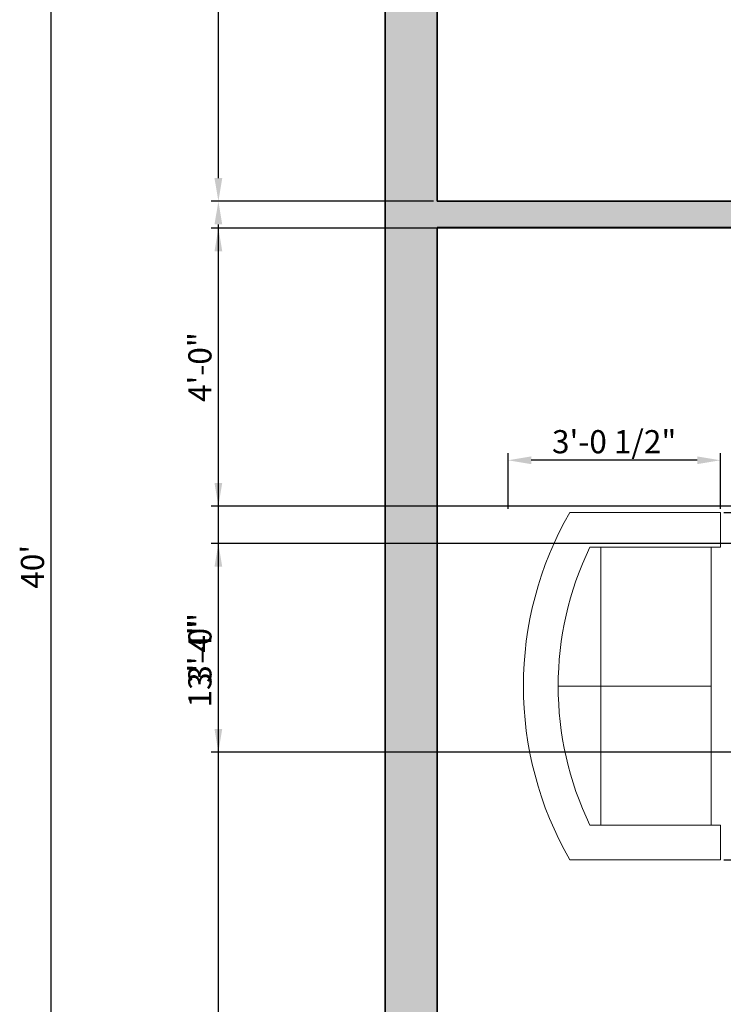
# Model space of a CAD drawing. Units: inches. Extents: x 1872 to 2380, y 714 to 1327.
# Tile 4 of 9: x 1872 to 1994, y 974 to 1144. Entities that reach past the tile are written whole.
import ezdxf

# ---------------------------------------------------------------- set-up
doc = ezdxf.new("R2010")
doc.units = ezdxf.units.IN
for name, color, linetype, lineweight in [('A-ANNO-DIMS', 2, 'Continuous', 18), ('A-FURN', 8, 'Continuous', 18), ('A-WALL', 7, 'Continuous', 35)]:
    doc.layers.add(name, color=color, linetype=linetype, lineweight=lineweight)
doc.layers.add('A-WALL-PATT', color=242, linetype='Continuous', lineweight=13, true_color=0xd52e31)
doc.styles.get("Standard").update_dxf_attribs({"font": 'arial.ttf'})
doc.dimstyles.new('ISO-25', dxfattribs={"dimtxt": 4, "dimasz": 4, "dimexe": 1.25, "dimexo": 0.625, "dimtad": 1, "dimdec": 0, "dimlunit": 3, "dimtxsty": 'Standard', "dimcen": 2.5, "dimadec": 0, "dimazin": 0, "dimtfac": 1, "dimtdec": 0, "dimtmove": 0, "dimatfit": 3, "dimfxl": 1, "dimarcsym": 0})

# ---------------------------------------------------------------- blocks, each defined once
blk = doc.blocks.new('Sofa - Roundback Loveseat 5 ft.')
for p, q in [((0, -32.44198), (0, -5.99998)), ((-24, -33.99998), (-24, -11.46958)), ((24.00004, -33.99998), (24.00004, -11.46958)), ((-23.9998, -13.38178), (23.99986, -13.38178)), ((-24, -32.44198), (24.00004, -32.44198))]:
    blk.add_line(p, q)
for points in [[(-24, -33.99998), (-30, -33.99998), (-30, -7.99998)], [(30.00004, -7.99998), (30.00004, -33.99998), (24.00004, -33.99998)]]:
    blk.add_lwpolyline(points)
for centre, radius, start, end in [((0, -60.24998), 60.24998, 60.13715, 119.8628), ((0, -61.38438), 55.38444, 64.32083, 115.6792)]:
    blk.add_arc(centre, radius, start, end)
blk = doc.blocks.new('*D23')
at = {"layer": 'A-ANNO-DIMS', "color": 0, "lineweight": -2, "transparency": 16777216}
for p, q in [((1934.77, 1289.64), (1876.44, 1289.64)), ((1877.69, 1285.64), (1877.69, 813.64)), ((1934.77, 809.64), (1876.44, 809.64))]:
    blk.add_line(p, q, dxfattribs=at)
at = {"layer": 'A-ANNO-DIMS', "color": 0, "transparency": 16777216}
for points in [[(1877.02, 1285.64), (1878.36, 1285.64), (1877.69, 1289.64)], [(1877.02, 813.64), (1878.36, 813.64), (1877.69, 809.64)]]:
    blk.add_solid(points, dxfattribs=at)
at = {"layer": 'Defpoints', "color": 0, "transparency": 16777216}
for p in [(1935.4, 1289.64), (1877.69, 809.64), (1935.4, 809.64)]:
    blk.add_point(p, dxfattribs=at)
at = {"layer": 'A-ANNO-DIMS', "color": 0, "transparency": 16777216, "insert": (1875.02, 1049.64), "char_height": 4, "attachment_point": 5, "rotation": 90}
blk.add_mtext("40'", dxfattribs=at)
blk = doc.blocks.new('*D40')
at = {"layer": 'A-ANNO-DIMS', "color": 0, "lineweight": -2, "transparency": 16777216}
for p, q in [((1993.9, 1059.04), (2003.52, 1059.04)), ((2002.27, 1003.04), (2002.27, 1055.04)), ((1993.9, 999.04), (2003.52, 999.04))]:
    blk.add_line(p, q, dxfattribs=at)
at = {"layer": 'A-ANNO-DIMS', "color": 0, "transparency": 16777216}
for points in [[(2001.61, 1055.04), (2002.94, 1055.04), (2002.27, 1059.04)], [(2001.61, 1003.04), (2002.94, 1003.04), (2002.27, 999.04)]]:
    blk.add_solid(points, dxfattribs=at)
at = {"layer": 'Defpoints', "color": 0, "transparency": 16777216}
for p in [(1993.27, 1059.04), (2002.27, 1059.04), (1993.27, 999.04)]:
    blk.add_point(p, dxfattribs=at)
at = {"layer": 'A-ANNO-DIMS', "color": 0, "transparency": 16777216, "insert": (1999.58, 1029.04), "char_height": 4, "attachment_point": 5, "rotation": 90}
blk.add_mtext('LOVESEAT 5\'-0"', dxfattribs=at)
blk = doc.blocks.new('*D41')
at = {"layer": 'A-ANNO-DIMS', "color": 0, "lineweight": -2, "transparency": 16777216}
for p, q in [((1956.61, 1059.66), (1956.61, 1069.29)), ((1993.27, 1059.66), (1993.27, 1069.29)), ((1989.27, 1068.04), (1960.61, 1068.04))]:
    blk.add_line(p, q, dxfattribs=at)
at = {"layer": 'A-ANNO-DIMS', "color": 0, "transparency": 16777216}
for points in [[(1960.61, 1068.71), (1960.61, 1067.37), (1956.61, 1068.04)], [(1989.27, 1068.71), (1989.27, 1067.37), (1993.27, 1068.04)]]:
    blk.add_solid(points, dxfattribs=at)
at = {"layer": 'Defpoints', "color": 0, "transparency": 16777216}
for p in [(1956.61, 1068.04), (1956.61, 1059.04), (1993.27, 1059.04)]:
    blk.add_point(p, dxfattribs=at)
at = {"layer": 'A-ANNO-DIMS', "color": 0, "transparency": 16777216, "insert": (1974.94, 1070.73), "char_height": 4, "attachment_point": 5}
blk.add_mtext('3\'-0 1/2"', dxfattribs=at)
blk = doc.blocks.new('*D67')
at = {"layer": 'A-ANNO-DIMS', "color": 0, "lineweight": -2, "transparency": 16777216}
for p, q in [((1943.77, 1112.77), (1905.35, 1112.77)), ((1906.6, 956.99), (1906.6, 1108.77)), ((2000.77, 952.99), (1905.35, 952.99))]:
    blk.add_line(p, q, dxfattribs=at)
at = {"layer": 'A-ANNO-DIMS', "color": 0, "transparency": 16777216}
for points in [[(1905.93, 1108.77), (1907.27, 1108.77), (1906.6, 1112.77)], [(1905.93, 956.99), (1907.27, 956.99), (1906.6, 952.99)]]:
    blk.add_solid(points, dxfattribs=at)
at = {"layer": 'Defpoints', "color": 0, "transparency": 16777216}
for p in [(1906.6, 1112.77), (1944.4, 1112.77), (2001.4, 952.99)]:
    blk.add_point(p, dxfattribs=at)
at = {"layer": 'A-ANNO-DIMS', "color": 0, "transparency": 16777216, "insert": (1903.93, 1032.88), "char_height": 4, "attachment_point": 5, "rotation": 90}
blk.add_mtext('13\'-4"', dxfattribs=at)
blk = doc.blocks.new('*D68')
at = {"layer": 'A-ANNO-DIMS', "color": 0, "lineweight": -2, "transparency": 16777216}
for p, q in [((1934.77, 1289.64), (1905.35, 1289.64)), ((1906.6, 1116.77), (1906.6, 1285.64)), ((1943.77, 1112.77), (1905.35, 1112.77))]:
    blk.add_line(p, q, dxfattribs=at)
at = {"layer": 'A-ANNO-DIMS', "color": 0, "transparency": 16777216}
for points in [[(1905.93, 1285.64), (1907.27, 1285.64), (1906.6, 1289.64)], [(1905.93, 1116.77), (1907.27, 1116.77), (1906.6, 1112.77)]]:
    blk.add_solid(points, dxfattribs=at)
at = {"layer": 'Defpoints', "color": 0, "transparency": 16777216}
for p in [(1906.6, 1289.64), (1935.4, 1289.64), (1944.4, 1112.77)]:
    blk.add_point(p, dxfattribs=at)
at = {"layer": 'A-ANNO-DIMS', "color": 0, "transparency": 16777216, "insert": (1903.93, 1201.21), "char_height": 4, "attachment_point": 5, "rotation": 90}
blk.add_mtext('14\'-9"', dxfattribs=at)
blk = doc.blocks.new('*D72')
at = {"layer": 'A-ANNO-DIMS', "color": 0, "lineweight": -2, "transparency": 16777216}
for p, q in [((2197.27, 1108.14), (1905.35, 1108.14)), ((1906.6, 1064.14), (1906.6, 1104.14)), ((2197.27, 1060.14), (1905.35, 1060.14))]:
    blk.add_line(p, q, dxfattribs=at)
at = {"layer": 'A-ANNO-DIMS', "color": 0, "transparency": 16777216}
for points in [[(1905.93, 1104.14), (1907.27, 1104.14), (1906.6, 1108.14)], [(1905.93, 1064.14), (1907.27, 1064.14), (1906.6, 1060.14)]]:
    blk.add_solid(points, dxfattribs=at)
at = {"layer": 'Defpoints', "color": 0, "transparency": 16777216}
for p in [(1906.6, 1108.14), (2197.9, 1108.14), (2197.9, 1060.14)]:
    blk.add_point(p, dxfattribs=at)
at = {"layer": 'A-ANNO-DIMS', "color": 0, "transparency": 16777216, "insert": (1903.93, 1084.14), "char_height": 4, "attachment_point": 5, "rotation": 90}
blk.add_mtext('4\'-0"', dxfattribs=at)
blk = doc.blocks.new('*D73')
at = {"layer": 'A-ANNO-DIMS', "color": 0, "lineweight": -2, "transparency": 16777216}
for p, q in [((2197.27, 1053.64), (1905.35, 1053.64)), ((1906.6, 1021.64), (1906.6, 1049.64)), ((2197.27, 1017.64), (1905.35, 1017.64))]:
    blk.add_line(p, q, dxfattribs=at)
at = {"layer": 'A-ANNO-DIMS', "color": 0, "transparency": 16777216}
for points in [[(1905.93, 1049.64), (1907.27, 1049.64), (1906.6, 1053.64)], [(1905.93, 1021.64), (1907.27, 1021.64), (1906.6, 1017.64)]]:
    blk.add_solid(points, dxfattribs=at)
at = {"layer": 'Defpoints', "color": 0, "transparency": 16777216}
for p in [(1906.6, 1053.64), (2197.9, 1053.64), (2197.9, 1017.64)]:
    blk.add_point(p, dxfattribs=at)
at = {"layer": 'A-ANNO-DIMS', "color": 0, "transparency": 16777216, "insert": (1903.93, 1035.64), "char_height": 4, "attachment_point": 5, "rotation": 90}
blk.add_mtext('3\'-0"', dxfattribs=at)

msp = doc.modelspace()

# ---------------------------------------------------------------- hatches: boundary and pattern name
at = {"layer": 'A-WALL-PATT', "transparency": 33554687}
h = msp.add_hatch(color=256, dxfattribs=at)
h.dxf.hatch_style = 1
h.paths.add_polyline_path([(2295.4, 1289.64), (1935.4, 1289.64), (1935.4, 809.64), (1949.4, 809.64), (1949.4, 818.64), (1944.4, 818.64), (1944.4, 1108.27), (2100.4, 1108.27), (2100.4, 1112.77), (1944.4, 1112.77), (1944.4, 1280.64), (2095.9, 1280.64), (2095.9, 1141.77), (2100.4, 1141.77), (2100.4, 1280.64), (2169.91, 1280.64), (2169.91, 1244.64), (2169.91, 1160.49, -0.053008), (2170.04, 1158.75, -0.03687), (2169.91, 1157.54), (2169.91, 1148.64), (2167.91, 1148.64), (2138.4, 1148.64), (2138.4, 1144.14), (2167.91, 1144.14), (2174.41, 1144.14), (2174.41, 1280.64), (2197.9, 1280.64), (2197.9, 1184.64), (2202.4, 1184.64), (2202.4, 1280.64), (2286.4, 1280.64), (2286.4, 1148.64), (2197.9, 1148.64), (2197.9, 1108.14), (2202.4, 1108.14), (2202.4, 1144.14), (2286.4, 1144.14), (2286.4, 1060.14), (2202.4, 1060.14), (2202.4, 1108.14), (2197.9, 1108.14), (2197.9, 1060.14), (2197.9, 1053.64), (2202.4, 1053.64), (2202.4, 1055.64), (2286.4, 1055.64), (2286.4, 976.14), (2202.4, 976.14), (2202.4, 1015.64), (2197.9, 1015.64), (2197.9, 971.64), (2197.9, 952.99), (2197.9, 818.64), (2101.9, 818.64), (2101.9, 948.71), (2130.4, 948.71), (2130.4, 952.99), (2073.4, 952.99), (2073.4, 948.71), (2097.4, 948.71), (2097.4, 818.64), (2005.9, 818.64), (2005.9, 948.71), (2029.9, 948.71), (2029.9, 952.99), (2001.4, 952.99), (2001.4, 818.64), (1996.4, 818.64), (1985.23, 818.64), (1985.23, 809.64), (1996.4, 809.64), (2295.4, 809.64)])
h.paths.add_polyline_path([(2202.4, 971.64), (2286.4, 971.64), (2286.4, 858.19), (2286.62, 858.19), (2286.62, 857.19), (2286.4, 857.19), (2286.4, 828.68), (2286.48, 828.76), (2286.4, 828.43), (2286.4, 818.64), (2256.29, 818.64), (2255.29, 818.39), (2254.54, 818.64), (2238.99, 818.64), (2238.75, 818.58), (2238.56, 818.64), (2202.4, 818.64), (2202.4, 952.99)], flags=16)
h.paths.add_polyline_path([(2260.41, 970, -0.15), (2280.41, 970), (2278.41, 967, 0.001913), (2277.92, 967.06), (2277.41, 964.5), (2278.64, 964.5), (2278.72, 964), (2279.41, 964), (2282.41, 953, -0.541163), (2280.76, 950.93), (2280.91, 950, -0.414214), (2279.91, 949), (2279.41, 949), (2279.91, 945), (2278.41, 945), (2277.91, 949), (2270.41, 949), (2262.91, 949), (2262.41, 945), (2260.91, 945), (2261.41, 949), (2260.91, 949, -0.414214), (2259.91, 950), (2260.05, 950.93, -0.505809), (2258.36, 952.83), (2261.41, 964), (2262.1, 964), (2262.17, 964.5), (2263.41, 964.5), (2262.9, 967.06, 0.001913), (2262.41, 967)], flags=0)
h.paths.add_polyline_path([(2257.85, 934.42), (2280.51, 934.42, -0.333333), (2281.77, 933.16), (2281.77, 923.09, -0.333333), (2280.51, 921.83), (2277.57, 921.83), (2277.57, 921.41), (2275.89, 921.41), (2275.89, 921.83), (2262.46, 921.83), (2262.46, 921.41), (2260.79, 921.41), (2260.79, 921.83), (2257.85, 921.83, -0.333333), (2256.59, 923.09), (2256.59, 933.16, -0.333333)], flags=0)
h.paths.add_polyline_path([(2260.61, 912.79), (2262.11, 912.79), (2262.61, 908.79), (2270.11, 908.79), (2277.61, 908.79), (2278.11, 912.79), (2279.61, 912.79), (2279.11, 908.79), (2279.61, 908.79, -0.414214), (2280.61, 907.79), (2280.46, 906.86, -0.505809), (2282.15, 904.96), (2279.11, 893.79), (2278.42, 893.79), (2278.34, 893.29), (2277.11, 893.29), (2277.62, 890.73, 0.001913), (2278.11, 890.79), (2280.11, 887.79, -0.15), (2260.11, 887.79), (2262.11, 890.79, 0.001913), (2262.59, 890.73), (2263.11, 893.29), (2261.87, 893.29), (2261.79, 893.79), (2261.11, 893.79), (2258.11, 904.79, -0.541163), (2259.75, 906.86), (2259.61, 907.79, -0.414214), (2260.61, 908.79), (2261.11, 908.79)], flags=0)
h.paths.add_polyline_path([(2252.62, 864.69), (2253.62, 864.69), (2253.62, 862.19), (2253.62, 860.69), (2256.62, 859.69, -0.362186), (2259.62, 862.19, -0.174416), (2262.62, 860.69, 0.103487), (2265.62, 859.19, -0.219276), (2266.55, 858.19), (2268.62, 858.19), (2268.62, 859.69), (2267.62, 859.69), (2267.62, 863.69), (2270.12, 863.69), (2270.12, 859.69), (2269.12, 859.69), (2269.12, 858.19), (2274.62, 858.19), (2278.62, 858.19), (2278.62, 862.69), (2275.62, 864.69), (2275.62, 865.69), (2279.62, 862.69), (2279.62, 858.19), (2279.62, 852.69), (2275.62, 849.19), (2275.62, 850.19), (2278.62, 852.69), (2278.62, 857.19), (2274.62, 857.19), (2271.12, 857.19), (2271.12, 855.69), (2272.12, 855.69), (2272.12, 851.69), (2269.62, 851.69), (2269.62, 855.69), (2270.62, 855.69), (2270.62, 857.19), (2266.55, 857.19, -0.219162), (2265.62, 856.19, 0.103506), (2262.62, 854.69, -0.174459), (2259.62, 853.19, -0.362114), (2256.62, 855.69), (2253.62, 854.69), (2253.62, 850.69), (2252.62, 850.69)], flags=0)
h.paths.add_polyline_path([(2253.62, 859.69), (2256.62, 858.69), (2256.62, 856.69), (2253.62, 855.69)], flags=0)
h.paths.add_polyline_path([(2208.62, 838.17), (2208.28, 836.61), (2207.75, 836.18), (2207.67, 833.93), (2208.71, 832.96), (2211.55, 836.09), (2214.43, 837.53), (2214.45, 837.55), (2214.61, 836.16), (2215.48, 834.9), (2215.87, 835.13), (2217.12, 836.79), (2216.83, 834.17), (2218.8, 828.76), (2219.23, 829.13), (2220.06, 831.53), (2219.5, 837.61), (2219.53, 837.66), (2219.68, 838.72), (2219.62, 838.91), (2219.72, 839.01), (2219.51, 837.47), (2219.77, 834.68), (2220.87, 834.05), (2221.03, 834.58), (2222.05, 835.47), (2222.71, 834.65), (2223.67, 836.89), (2224.63, 836.57), (2226.23, 835.08), (2227.55, 836.18), (2227.59, 837.16), (2228.42, 838.17), (2228.08, 836.61), (2227.55, 836.18), (2227.47, 833.93), (2228.51, 832.96), (2231.35, 836.09), (2234.23, 837.53), (2234.25, 837.55), (2234.42, 836.16), (2235.28, 834.9), (2235.67, 835.13), (2236.93, 836.79), (2236.93, 836.84), (2238.69, 834.65), (2239.41, 836.34), (2239.3, 837.61), (2239.34, 837.66), (2239.48, 838.72), (2239.42, 838.91), (2239.52, 839.01), (2239.31, 837.47), (2239.36, 836.98), (2240.61, 836.57), (2242.2, 835.08), (2243.53, 836.18), (2243.57, 837.16), (2244.39, 838.17), (2244.05, 836.61), (2243.53, 836.18), (2243.44, 833.93), (2244.49, 832.96), (2247.33, 836.09), (2250.21, 837.53), (2250.22, 837.55), (2250.39, 836.16), (2251.25, 834.9), (2251.65, 835.13), (2252.9, 836.79), (2252.61, 834.17), (2254.09, 830.08), (2254.54, 829.37), (2254.85, 828.99), (2255.01, 829.13), (2255.83, 831.53), (2255.29, 837.44), (2255.28, 837.44), (2255.46, 838.72), (2255.4, 838.91), (2255.5, 839.01), (2255.28, 837.47), (2255.29, 837.44), (2257.9, 836.57), (2259.5, 835.08), (2260.82, 836.18), (2260.86, 837.16), (2261.69, 838.17), (2261.35, 836.61), (2260.82, 836.18), (2260.74, 833.93), (2261.78, 832.96), (2264.62, 836.09), (2267.5, 837.53), (2267.52, 837.55), (2267.68, 836.16), (2268.54, 834.9), (2268.94, 835.13), (2270.19, 836.79), (2269.9, 834.17), (2271.79, 828.96), (2271.98, 828.86), (2272.3, 829.13), (2273.13, 831.53), (2272.56, 837.61), (2272.6, 837.66), (2272.75, 838.72), (2272.69, 838.91), (2272.79, 839.01), (2272.58, 837.47), (2273.13, 831.53), (2273.02, 831.22), (2273.67, 831.01), (2273.92, 831.6), (2273.83, 830.95), (2274.1, 830.86), (2275.75, 833.35), (2276.03, 831.86), (2276.57, 831.38), (2277, 831.91), (2277.3, 833.27), (2279.06, 830.44), (2281.09, 831.46), (2281.1, 831.48), (2281.21, 830.5), (2281.82, 829.61), (2282.1, 829.77), (2282.98, 830.94), (2282.77, 829.1), (2284.15, 825.3), (2284.46, 825.55), (2285.04, 827.24), (2284.64, 831.51), (2284.67, 831.55), (2284.77, 832.3), (2284.73, 832.43), (2284.8, 832.5), (2284.65, 831.42), (2285.04, 827.24), (2284.46, 825.55), (2283.45, 824.71), (2281.76, 819.99), (2278.73, 818.64), (2276.7, 819.65), (2275.69, 821.34), (2274.34, 822.01), (2272.32, 824.04), (2269.58, 824.33), (2268.46, 821.21), (2264.14, 819.29), (2261.26, 820.73), (2259.82, 823.13), (2257.9, 824.09), (2255.02, 826.97), (2253.29, 827.15), (2251.17, 821.21), (2246.85, 819.29), (2243.97, 820.73), (2242.53, 823.13), (2240.61, 824.09), (2237.73, 826.97), (2237.27, 827.01), (2235.19, 821.21), (2230.87, 819.29), (2227.99, 820.73), (2226.55, 823.13), (2224.63, 824.09), (2221.75, 826.97), (2217.61, 827.41), (2215.39, 821.21), (2211.07, 819.29), (2208.19, 820.73), (2206.75, 823.13), (2204.83, 824.09), (2203.87, 826.49), (2202.91, 830.81), (2202.91, 834.65), (2203.87, 836.89), (2204.83, 836.57), (2206.43, 835.08), (2207.75, 836.18), (2207.79, 837.16)], flags=0)
h.paths.add_polyline_path([(2221.04, 832.88), (2221.82, 832.52), (2222.11, 833.69), (2222.71, 834.29), (2222.71, 832.11), (2225.59, 830.81), (2226.55, 830.81), (2228.95, 822.65), (2230.87, 820.25), (2230.87, 819.29), (2233.27, 821.21), (2233.75, 823.61), (2232.79, 826.97), (2231.99, 830.19), (2236.41, 827.71), (2236.63, 831.29), (2235.93, 834.58), (2242.53, 830.81), (2241.57, 830.81), (2240.97, 831.07), (2240.47, 830.33), (2239.06, 829.14), (2239.65, 826.49), (2237.25, 829.37), (2236.52, 829.55), (2236.41, 827.71), (2231.99, 830.19), (2232.79, 826.97), (2233.75, 823.61), (2233.27, 821.21), (2230.87, 819.29), (2230.87, 820.25), (2228.95, 822.65), (2226.55, 830.81), (2225.59, 830.81), (2222.71, 832.11), (2222.71, 830.81), (2223.67, 826.49), (2221.27, 829.37), (2220.67, 830.33), (2220.67, 830.33)], flags=0)
h.paths.add_polyline_path([(2255.98, 833), (2259.82, 830.81), (2258.86, 830.81), (2257.25, 831.54), (2256.45, 830.33), (2256.66, 831.81), (2256.02, 832.1), (2255.98, 831.99)], flags=0)
h.paths.add_polyline_path([(2275.69, 826.73), (2277.07, 828.25), (2275.46, 829.74), (2276.39, 830.51), (2276.33, 828.93), (2279.06, 826.4), (2278.73, 823.36), (2277.38, 821)], flags=0)
h.paths.add_polyline_path([(2260.6, 925.25), (2276.34, 925.25), (2276.34, 931.01), (2260.6, 931.01)], flags=8)
h.paths.add_polyline_path([(2202.72, 1070.05), (2202.72, 1092.72), (2197.34, 1092.72), (2197.34, 1070.05)], flags=25)

# ---------------------------------------------------------------- linework, layer by layer
at = {"layer": 'A-WALL', "transparency": 33554687}
msp.add_line((1944.4, 1112.77), (1944.4, 1280.64), dxfattribs=at)
at = {"layer": 'A-WALL'}
for p, q in [((1944.4, 1112.77), (2100.4, 1112.77)), ((1944.4, 818.64), (1944.4, 1108.27)), ((1944.4, 1108.27), (2100.4, 1108.27))]:
    msp.add_line(p, q, dxfattribs=at)
at = {"layer": 'A-WALL', "transparency": 33554687}
msp.add_lwpolyline([(1949.4, 809.64), (1935.4, 809.64), (1935.4, 1289.64), (2295.4, 1289.64), (2295.4, 809.64), (1996.4, 809.64)], dxfattribs=at)

# ---------------------------------------------------------------- block references
at = {"layer": 'A-FURN', "transparency": 33554687, "rotation": 90}
msp.add_blockref('Sofa - Roundback Loveseat 5 ft.', (1959.27, 1029.04), dxfattribs=at)

# ---------------------------------------------------------------- dimensions: what is measured, and where the dimension line sits
at = {"layer": 'A-ANNO-DIMS', "transparency": 33554687}
for base, p1, p2, angle, override, picture, middle in [((1877.69, 809.64), (1935.4, 1289.64), (1935.4, 809.64), 90, {"dimclrd": 0, "dimclre": 0, "dimclrt": 0}, '*D23', (1875.02, 1049.64)), ((1906.6, 1289.64), (1944.4, 1112.77), (1935.4, 1289.64), 90, {"dimdec": 1, "dimlfac": 1, "dimrnd": 0, "dimzin": 1, "dimdsep": 46, "dimlunit": 4, "dimfrac": 2}, '*D68', (1903.93, 1201.21)), ((1906.6, 1112.77), (2001.4, 952.99), (1944.4, 1112.77), 90, {"dimdec": 1, "dimlfac": 1, "dimrnd": 0, "dimzin": 1, "dimdsep": 46, "dimlunit": 4, "dimfrac": 2}, '*D67', (1903.93, 1032.88)), ((1906.6, 1108.14), (2197.9, 1060.14), (2197.9, 1108.14), 90, {"dimdec": 1, "dimlfac": 1, "dimrnd": 0, "dimzin": 1, "dimdsep": 46, "dimlunit": 4, "dimfrac": 2}, '*D72', (1903.93, 1084.14)), ((1956.61, 1068.04), (1993.27, 1059.04), (1956.61, 1059.04), 180, {"dimdec": 1, "dimlfac": 1, "dimrnd": 0, "dimzin": 1, "dimdsep": 46, "dimlunit": 4, "dimfrac": 2}, '*D41', (1974.94, 1070.73)), ((1906.6, 1053.64), (2197.9, 1017.64), (2197.9, 1053.64), 90, {"dimdec": 1, "dimlfac": 1, "dimrnd": 0, "dimzin": 1, "dimdsep": 46, "dimlunit": 4, "dimfrac": 2}, '*D73', (1903.93, 1035.64))]:
    dim = msp.add_linear_dim(base=base, p1=p1, p2=p2, angle=angle, dimstyle='ISO-25', override=override, dxfattribs=at)
    dim.commit()
    dim.dimension.update_dxf_attribs({"geometry": picture, "text_midpoint": middle})
dim = msp.add_linear_dim(base=(2002.27, 1059.04), p1=(1993.27, 999.04), p2=(1993.27, 1059.04), angle=90, text='LOVESEAT <>', dimstyle='ISO-25', override={"dimdec": 1, "dimlfac": 1, "dimrnd": 0, "dimzin": 1, "dimdsep": 46, "dimlunit": 4, "dimfrac": 2}, dxfattribs=at)
dim.commit()
dim.dimension.update_dxf_attribs({"geometry": '*D40', "text_midpoint": (1999.58, 1029.04)})

doc.saveas('drawing.dxf')
